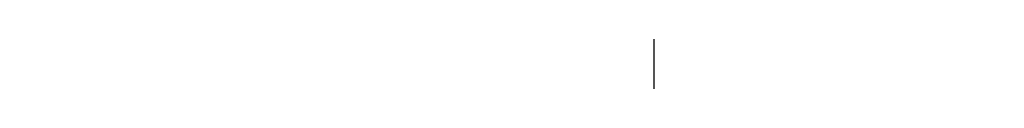
# Model space of a CAD drawing. Units: inches. Extents: x 2083 to 3317, y 1141 to 2115.
# Tile 64 of 256: x 2237.106 to 2238.294, y 1477.8 to 1477.842. Entities that reach past the tile are written whole.
import ezdxf

# ---------------------------------------------------------------- set-up
doc = ezdxf.new("R2010")
doc.units = ezdxf.units.IN
doc.layers.add('A-ANNO-DIMS', color=2, linetype='Continuous', lineweight=18)
doc.layers.add('A-WALL-PATT', color=251, linetype='Continuous', lineweight=13, true_color=0x636466)
doc.styles.get("Standard").update_dxf_attribs({"font": 'arial.ttf'})
doc.dimstyles.new('ISO-25', dxfattribs={"dimtxt": 12, "dimasz": 12, "dimexe": 1.25, "dimexo": 0.625, "dimtad": 1, "dimlunit": 3, "dimtxsty": 'Standard', "dimcen": 2.5, "dimadec": 0, "dimazin": 0, "dimtfac": 1, "dimtmove": 0, "dimatfit": 3, "dimfxl": 1, "dimarcsym": 0})

# ---------------------------------------------------------------- blocks, each defined once
blk = doc.blocks.new('*D30')
at = {"layer": 'A-ANNO-DIMS', "color": 0, "lineweight": -2, "transparency": 16777216}
for p, q in [((2240.0179, 1445.2738), (2240.0179, 1448.0455)), ((2254.3293, 1445.2738), (2254.3293, 1448.0455)), ((2228.0179, 1446.7955), (2216.0179, 1446.7955)), ((2240.0179, 1446.7955), (2254.3293, 1446.7955)), ((2266.3293, 1446.7955), (2413.7649, 1446.7955))]:
    blk.add_line(p, q, dxfattribs=at)
at = {"layer": 'A-ANNO-DIMS', "color": 0, "transparency": 16777216}
for points in [[(2228.0179, 1448.7955), (2228.0179, 1444.7955), (2240.0179, 1446.7955)], [(2266.3293, 1448.7955), (2266.3293, 1444.7955), (2254.3293, 1446.7955)]]:
    blk.add_solid(points, dxfattribs=at)
at = {"layer": 'Defpoints', "color": 0, "transparency": 16777216}
for p in [(2254.3293, 1446.7955), (2240.0179, 1444.6488), (2254.3293, 1444.6488)]:
    blk.add_point(p, dxfattribs=at)
at = {"layer": 'A-ANNO-DIMS', "color": 0, "transparency": 16777216, "insert": (2346.0471, 1453.6252), "char_height": 12, "attachment_point": 5}
blk.add_mtext('WC 1\'-2 1/2" TYP.', dxfattribs=at)
blk = doc.blocks.new('*D31')
at = {"layer": 'A-ANNO-DIMS', "color": 0, "lineweight": -2, "transparency": 16777216}
for p, q in [((2237.8711, 1456.6488), (2237.8711, 1541.9152)), ((2239.3929, 1444.6488), (2236.6211, 1444.6488)), ((2237.8711, 1431.5475), (2237.8711, 1444.6488)), ((2239.3929, 1431.5475), (2236.6211, 1431.5475)), ((2237.8711, 1419.5475), (2237.8711, 1407.5475))]:
    blk.add_line(p, q, dxfattribs=at)
at = {"layer": 'A-ANNO-DIMS', "color": 0, "transparency": 16777216}
for points in [[(2235.8711, 1456.6488), (2239.8711, 1456.6488), (2237.8711, 1444.6488)], [(2235.8711, 1419.5475), (2239.8711, 1419.5475), (2237.8711, 1431.5475)]]:
    blk.add_solid(points, dxfattribs=at)
at = {"layer": 'Defpoints', "color": 0, "transparency": 16777216}
for p in [(2237.8711, 1444.6488), (2240.0179, 1444.6488), (2240.0179, 1431.5475)]:
    blk.add_point(p, dxfattribs=at)
at = {"layer": 'A-ANNO-DIMS', "color": 0, "transparency": 16777216, "insert": (2231.2175, 1505.282), "char_height": 12, "attachment_point": 5, "rotation": 90}
blk.add_mtext('1\'-1" TYP.', dxfattribs=at)
blk = doc.blocks.new('*D45')
at = {"layer": 'A-ANNO-DIMS', "color": 0, "lineweight": -2, "transparency": 16777216}
for p, q in [((2235.9598, 1478.3864), (2235.9598, 1531.3614)), ((2418.9598, 1478.3864), (2418.9598, 1531.3614)), ((2247.9598, 1530.1114), (2406.9598, 1530.1114))]:
    blk.add_line(p, q, dxfattribs=at)
at = {"layer": 'A-ANNO-DIMS', "color": 0, "transparency": 16777216}
for points in [[(2247.9598, 1532.1114), (2247.9598, 1528.1114), (2235.9598, 1530.1114)], [(2406.9598, 1532.1114), (2406.9598, 1528.1114), (2418.9598, 1530.1114)]]:
    blk.add_solid(points, dxfattribs=at)
at = {"layer": 'Defpoints', "color": 0, "transparency": 16777216}
for p in [(2418.9598, 1530.1114), (2235.9598, 1477.7614), (2418.9598, 1477.7614)]:
    blk.add_point(p, dxfattribs=at)
at = {"layer": 'A-ANNO-DIMS', "color": 0, "transparency": 16777216, "insert": (2327.4598, 1536.8673), "char_height": 12, "attachment_point": 5}
blk.add_mtext('15\'-3"', dxfattribs=at)
blk = doc.blocks.new('*D62')
at = {"layer": 'A-ANNO-DIMS', "color": 0, "lineweight": -2, "transparency": 16777216}
for p, q in [((2235.9598, 1469.3864), (2235.9598, 1522.3614)), ((2379.9598, 1469.3864), (2379.9598, 1522.3614)), ((2247.9598, 1521.1114), (2367.9598, 1521.1114))]:
    blk.add_line(p, q, dxfattribs=at)
at = {"layer": 'A-ANNO-DIMS', "color": 0, "transparency": 16777216}
for points in [[(2247.9598, 1523.1114), (2247.9598, 1519.1114), (2235.9598, 1521.1114)], [(2367.9598, 1523.1114), (2367.9598, 1519.1114), (2379.9598, 1521.1114)]]:
    blk.add_solid(points, dxfattribs=at)
at = {"layer": 'Defpoints', "color": 0, "transparency": 16777216}
for p in [(2379.9598, 1521.1114), (2235.9598, 1468.7614), (2379.9598, 1468.7614)]:
    blk.add_point(p, dxfattribs=at)
at = {"layer": 'A-ANNO-DIMS', "color": 0, "transparency": 16777216, "insert": (2307.9598, 1527.8632), "char_height": 12, "attachment_point": 5}
blk.add_mtext('12\'-0"', dxfattribs=at)

msp = doc.modelspace()

# ---------------------------------------------------------------- hatches: boundary and pattern name
at = {"layer": 'A-WALL-PATT'}
h = msp.add_hatch(color=256, dxfattribs=at)
h.dxf.hatch_style = 1
h.paths.add_polyline_path([(3126.9598, 2020.7614), (2748.9598, 2020.7614), (2604.9598, 2020.7614), (2226.9598, 2020.7614), (2226.9598, 1702.7614), (2466.9598, 1702.7614), (2466.9598, 1582.7614), (2418.9598, 1582.7614), (2418.9598, 1477.7614), (2226.9598, 1477.7614), (2226.9598, 1263.2614), (2544.9598, 1263.2614), (2544.9598, 1411.7614), (2604.9598, 1411.7614), (2685.9598, 1411.7614), (2685.9598, 1420.7614), (2604.9598, 1420.7614), (2604.9598, 1573.7614), (2604.9598, 1702.7614), (2604.9598, 2011.7614), (2748.9598, 2011.7614), (2748.9598, 1702.7614), (2862.9598, 1702.7614), (2862.9598, 1621.7614), (2871.9598, 1621.7614), (2871.9598, 1702.7614), (2883.9598, 1702.7614), (2883.9598, 1706.9395, -0.026459), (2883.9598, 1711.7614), (2757.9598, 1711.7614), (2757.9598, 1807.7614), (2787.9598, 1807.7614), (2787.9598, 1812.2614), (2757.9598, 1812.2614), (2757.9598, 2011.7614), (2877.9598, 2011.7614), (2877.9598, 1812.2614), (2847.9598, 1812.2614), (2847.9598, 1807.7614), (2889.8357, 1807.7614), (2889.8357, 1812.2614), (2882.4598, 1812.2614), (2882.4598, 2011.7614), (3117.9598, 2011.7614), (3117.9598, 1812.2614), (2937.8357, 1812.2614), (2937.8357, 1807.7614), (2995.7098, 1807.7614), (2995.7098, 1796.1177), (3000.2098, 1796.1177), (3000.2098, 1807.7614), (3117.9598, 1807.7614), (3117.9598, 1711.7614), (3000.2098, 1711.7614), (3000.2098, 1760.1177), (2998.5727, 1760.1177, -0.020711), (2995.7098, 1760.1177), (2995.7098, 1711.7614), (2931.9598, 1711.7614), (2931.9598, 1702.7614), (3126.9598, 1702.7614)])
h.paths.add_polyline_path([(2471.4598, 2011.7614), (2471.4598, 1810.0114), (2462.7169, 1810.0114), (2462.7169, 1805.5114), (2505.9598, 1805.5114), (2505.9598, 1810.0114), (2475.9598, 1810.0114), (2475.9598, 2011.7614), (2595.9598, 2011.7614), (2595.9598, 1810.0114), (2565.9598, 1810.0114), (2565.9598, 1805.5114), (2595.9598, 1805.5114), (2595.9598, 1711.7614), (2235.9598, 1711.7614), (2235.9598, 1805.5114), (2353.7098, 1805.5114), (2353.7098, 1796.0542), (2358.2098, 1796.0542), (2358.2098, 1805.5114), (2414.7169, 1805.5114), (2414.7169, 1810.0114), (2235.9598, 1810.0114), (2235.9598, 2011.7614)], flags=16)
h.paths.add_polyline_path([(2270.2047, 1994.61), (2270.2047, 1970.61), (2246.2047, 1970.61), (2246.2047, 1994.61)], flags=0)
edge = h.paths.add_edge_path(flags=0)
edge.add_ellipse((2332.0274, 1899.7982), major_axis=(-3.043, 3.043), ratio=0.168252, start_angle=-161.3322, end_angle=-156.3071, ccw=False)
edge.add_ellipse((2333.082, 1898.7435), major_axis=(-1.0546, 1.0546), ratio=0.453532, start_angle=-123.371, end_angle=-94.1591)
edge = h.paths.add_edge_path(flags=0)
edge.add_ellipse((2332.0274, 1968.8763), major_axis=(3.043, 3.043), ratio=0.168252, start_angle=18.6678, end_angle=23.6929)
edge.add_spline(control_points=[(2332.9256, 1970.6911), (2332.2268, 1970.3361), (2330.8937, 1969.6589), (2328.4131, 1970.9321), (2327.2039, 1967.7487), (2324.7096, 1969.9556), (2322.5328, 1967.0124), (2320.0128, 1971.2958), (2317.6803, 1968.1578), (2316.0405, 1967.102), (2315.4269, 1966.8096)], knot_values=[0, 0, 0, 0, 2.267059, 4.324559, 6.685584, 8.878641, 11.121502, 14.300359, 17.755284, 19.732645, 19.732645, 19.732645, 19.732645], degree=3, periodic=0)
edge.add_ellipse((2332.0274, 1968.8763), major_axis=(3.043, 3.043), ratio=0.168252, start_angle=18.6678, end_angle=23.6929, ccw=False)
edge.add_ellipse((2333.082, 1969.9309), major_axis=(1.0546, 1.0546), ratio=0.453532, start_angle=56.629, end_angle=85.8409, ccw=False)
edge = h.paths.add_edge_path(flags=0)
edge.add_spline(control_points=[(2296.4283, 1967.9879), (2293.6278, 1965.3363), (2287.7036, 1959.7271), (2299.7439, 1949.9957), (2294.5326, 1935.6685), (2290.5732, 1920.6035), (2293.3941, 1909.9737), (2296.1854, 1904.9665)], knot_values=[0.099185, 0.099185, 0.099185, 0.099185, 0.345301, 0.619822, 0.982653, 1.386093, 1.810555, 1.810555, 1.810555, 1.810555], degree=3, periodic=0)
edge.add_spline(control_points=[(2296.1854, 1904.9665), (2297.3836, 1902.6193), (2298.001, 1901.9493), (2298.553, 1901.4682)], knot_values=[0.006246, 0.006246, 0.006246, 0.006246, 0.055476, 0.055476, 0.055476, 0.055476], degree=3, periodic=0)
edge.add_spline(control_points=[(2298.553, 1901.4682), (2297.2586, 1900.9232), (2295.2253, 1900.2321), (2293.0602, 1900.6142), (2292.1014, 1900.7884), (2292.0896, 1900.7906)], knot_values=[0.312835, 0.312835, 0.312835, 0.312835, 0.40178, 0.474987, 0.475903, 0.475903, 0.475903, 0.475903], degree=3, periodic=0)
edge.add_arc((2292.7936, 1904.6641), 3.937, 215.4209, 259.6982, ccw=False)
edge.add_spline(control_points=[(2289.5853, 1902.3823), (2289.4767, 1902.5351), (2289.3685, 1902.688), (2289.2609, 1902.8412)], knot_values=[0.102872, 0.102872, 0.102872, 0.102872, 0.116896, 0.116896, 0.116896, 0.116896], degree=3, periodic=0)
edge.add_spline(control_points=[(2289.2609, 1902.8412), (2288.6866, 1902.5502), (2287.64, 1902.0199), (2285.8813, 1901.874), (2283.853, 1901.5044), (2281.72, 1899.7105), (2278.467, 1899.4929), (2276.1571, 1901.8832), (2272.259, 1899.8041), (2267.7776, 1901.8432), (2262.2439, 1900.184), (2257.4149, 1901.7821), (2254.3184, 1900.7261), (2253.1783, 1900.3373)], knot_values=[0, 0, 0, 0, 1.907977, 3.477176, 5.261074, 7.972851, 11.680248, 13.717921, 16.939592, 22.789562, 27.502503, 33.595215, 37.145618, 37.145618, 37.145618, 37.145618], degree=3, periodic=0)
edge.add_line((2253.1783, 1900.3373), (2250.2442, 1902.8412))
edge.add_line((2250.2442, 1902.8412), (2250.2442, 1965.8333))
edge.add_line((2250.2442, 1965.8333), (2253.1783, 1968.3371))
edge.add_spline(control_points=[(2253.1783, 1968.3371), (2254.3184, 1967.9483), (2257.4149, 1966.8924), (2262.2439, 1968.4904), (2267.7776, 1966.8313), (2271.5267, 1968.5372), (2273.8759, 1967.8283), (2274.2067, 1967.7276)], knot_values=[0, 0, 0, 0, 0.09018, 0.244935, 0.364644, 0.513233, 0.537855, 0.537855, 0.537855, 0.537855], degree=3, periodic=0)
edge.add_arc((2274.3529, 1963.7933), 3.937, 72.0511, 92.1279, ccw=False)
edge.add_arc((2281.2969, 1985.23), 18.5963, 252.05113, 288.56572)
edge.add_arc((2292.3167, 1956.0289), 12.6461, 71.02679, 113.77822, ccw=False)
edge = h.paths.add_edge_path(flags=0)
edge.add_spline(control_points=[(2274.8994, 1951.8562), (2275.0662, 1951.6166), (2275.2327, 1951.3766), (2275.398, 1951.1359)], knot_values=[1.409916, 1.409916, 1.409916, 1.409916, 1.43159, 1.43159, 1.43159, 1.43159], degree=3, periodic=0)
edge.add_spline(control_points=[(2275.398, 1951.1359), (2275.7921, 1950.5619), (2276.1792, 1949.9838), (2276.5455, 1949.3971)], knot_values=[1.358238, 1.358238, 1.358238, 1.358238, 1.409916, 1.409916, 1.409916, 1.409916], degree=3, periodic=0)
edge.add_line((2276.5455, 1949.3971), (2277.4373, 1947.8622))
edge.add_spline(control_points=[(2277.4373, 1947.8622), (2276.3038, 1945.6731), (2274.6397, 1942.4269), (2274.6316, 1938.0939), (2272.7991, 1930.8515), (2274.3564, 1943.897), (2275.9477, 1947.9234), (2276.5455, 1949.3971)], knot_values=[0.005632, 0.005632, 0.005632, 0.005632, 0.186014, 0.266002, 0.357087, 0.59639, 0.739732, 0.739732, 0.739732, 0.739732], degree=3, periodic=0)
edge.add_spline(control_points=[(2276.5455, 1949.3971), (2276.1792, 1949.9838), (2275.7921, 1950.5619), (2275.398, 1951.1359)], knot_values=[1.358238, 1.358238, 1.358238, 1.358238, 1.409916, 1.409916, 1.409916, 1.409916], degree=3, periodic=0)
edge.add_spline(control_points=[(2275.398, 1951.1359), (2274.9425, 1950.0805), (2274.2078, 1948.0253), (2273.9346, 1944.8515), (2272.4685, 1937.6275), (2273.4662, 1945.6965), (2274.7006, 1951.0595), (2274.8994, 1951.8562)], knot_values=[0.104364, 0.104364, 0.104364, 0.104364, 0.189636, 0.269624, 0.36071, 0.600013, 0.644622, 0.644622, 0.644622, 0.644622], degree=3, periodic=0)
h.paths.add_polyline_path([(2269.1675, 1963.1276, -0.357527), (2268.1706, 1960.9764, -0.092561), (2268.1706, 1939.4363, -0.357527), (2269.1675, 1937.2851, -0.357527), (2267.0163, 1938.282, -0.164785), (2254.6856, 1938.282, -0.357527), (2252.5344, 1937.2851, -0.357527), (2253.5313, 1939.4363, -0.092561), (2253.5313, 1960.9764, -0.357527), (2252.5344, 1963.1276, -0.357527), (2254.6856, 1962.1307, -0.164785), (2267.0163, 1962.1307, -0.357527)], flags=0)
h.paths.add_polyline_path([(2248.8741, 1967.8018), (2248.8741, 1957.0277), (2249.4578, 1957.0277), (2249.4578, 1911.6468), (2248.8741, 1911.6468), (2248.8741, 1900.8727), (2246.5119, 1900.8727, 0.197327), (2244.1497, 1902.4569), (2244.1497, 1966.2176, 0.197327), (2246.5119, 1967.8018)], flags=0)
h.paths.add_polyline_path([(2269.1675, 1931.3893, -0.357527), (2268.1706, 1929.2381, -0.092561), (2268.1706, 1907.6981, -0.357527), (2269.1675, 1905.5469, -0.357527), (2267.0163, 1906.5438, -0.164785), (2254.6856, 1906.5438, -0.357527), (2252.5344, 1905.5469, -0.357527), (2253.5313, 1907.6981, -0.092561), (2253.5313, 1929.2381, -0.357527), (2252.5344, 1931.3893, -0.357527), (2254.6856, 1930.3925, -0.164785), (2267.0163, 1930.3925, -0.357527)], flags=0)
edge = h.paths.add_edge_path(flags=0)
edge.add_spline(control_points=[(2276.1969, 1906.7237), (2276.1681, 1909.0289), (2276.114, 1913.3719), (2270.5984, 1924.925), (2273.9052, 1919.0128), (2275.9217, 1916.2621), (2275.4746, 1912.4021), (2277.2579, 1910.3806), (2276.696, 1908.225), (2276.6462, 1906.813), (2276.6178, 1906.0084)], knot_values=[0, 0, 0, 0, 8.61026, 16.221274, 18.843057, 23.804898, 27.440828, 29.356102, 31.203478, 33.650687, 33.650687, 33.650687, 33.650687], degree=3, periodic=0)
edge.add_spline(control_points=[(2276.6178, 1906.0084), (2276.6233, 1905.6241), (2276.4977, 1904.6287), (2275.4418, 1903.8547), (2274.9373, 1903.0804), (2274.8591, 1902.8412)], knot_values=[0.156488, 0.156488, 0.156488, 0.156488, 0.184398, 0.231376, 0.250598, 0.250598, 0.250598, 0.250598], degree=3, periodic=0)
edge.add_line((2274.8591, 1902.8412), (2276.506, 1902.8412))
edge.add_spline(control_points=[(2276.506, 1902.8412), (2276.7883, 1903.0849), (2277.6651, 1904.1252), (2278.2495, 1904.3407), (2277.6539, 1908.5274), (2278.1557, 1906.2278), (2278.1005, 1905.2859), (2278.8467, 1904.069), (2277.8568, 1903.4149), (2277.8742, 1902.991), (2277.9036, 1902.8412)], knot_values=[0.059574, 0.059574, 0.059574, 0.059574, 0.080753, 0.103741, 0.16972, 0.176036, 0.207137, 0.240474, 0.262341, 0.27366, 0.27366, 0.27366, 0.27366], degree=3, periodic=0)
edge.add_line((2277.9036, 1902.8412), (2280.0298, 1902.8412))
edge.add_spline(control_points=[(2280.0298, 1902.8412), (2279.8882, 1903.0884), (2279.4993, 1903.9816), (2280.1523, 1905.9393), (2278.1036, 1909.6578), (2279.7624, 1907.1853), (2280.3279, 1904.8749), (2280.4851, 1903.4896), (2281.4633, 1903.2494), (2281.7583, 1902.9365), (2281.834, 1902.8412)], knot_values=[0.013856, 0.013856, 0.013856, 0.013856, 0.034874, 0.088867, 0.107879, 0.126738, 0.158714, 0.193757, 0.217487, 0.226722, 0.226722, 0.226722, 0.226722], degree=3, periodic=0)
edge.add_spline(control_points=[(2281.834, 1902.8412), (2281.7875, 1902.8267), (2281.647, 1902.783), (2281.3955, 1902.8595), (2281.0881, 1902.9852), (2280.7207, 1903.0609), (2280.3335, 1903.0257), (2280.1248, 1902.8989), (2280.0298, 1902.8412)], knot_values=[0, 0, 0, 0, 0.14413, 0.435517, 0.749276, 1.153046, 1.548371, 1.878348, 1.878348, 1.878348, 1.878348], degree=3, periodic=0)
edge.add_line((2280.0298, 1902.8412), (2277.9036, 1902.8412))
edge.add_spline(control_points=[(2277.9036, 1902.8412), (2277.8929, 1902.7959), (2277.8654, 1902.6796), (2277.6075, 1902.6875), (2277.2741, 1902.8007), (2276.8379, 1902.6198), (2276.5838, 1902.7893), (2276.506, 1902.8412)], knot_values=[0, 0, 0, 0, 0.127189, 0.326199, 0.628009, 1.24357, 1.515331, 1.515331, 1.515331, 1.515331], degree=3, periodic=0)
edge.add_line((2276.506, 1902.8412), (2274.8591, 1902.8412))
edge.add_spline(control_points=[(2274.8591, 1902.8412), (2274.8144, 1902.8986), (2274.7251, 1903.0134), (2274.4935, 1903.119), (2274.2443, 1902.9605), (2273.9371, 1903.1849), (2273.614, 1902.9831), (2273.4083, 1902.883), (2273.3223, 1902.8412)], knot_values=[0, 0, 0, 0, 0.21843, 0.436957, 0.687977, 0.990379, 1.398396, 1.69185, 1.69185, 1.69185, 1.69185], degree=3, periodic=0)
edge.add_spline(control_points=[(2273.3223, 1902.8412), (2273.6167, 1903.4457), (2274.274, 1904.5383), (2276.0272, 1904.5737), (2276.207, 1906.5836), (2276.1969, 1906.7237)], knot_values=[0.012227, 0.012227, 0.012227, 0.012227, 0.059472, 0.106218, 0.134458, 0.134458, 0.134458, 0.134458], degree=3, periodic=0)
h.paths.add_polyline_path([(2270.7761, 1897.7898), (2270.7761, 1873.7898), (2246.7761, 1873.7898), (2246.7761, 1897.7898)], flags=0)
h.paths.add_polyline_path([(2353.7098, 1760.0051), (2353.7098, 1760.0542), (2358.2098, 1760.0542, -0.033729)], flags=0)
h.paths.add_polyline_path([(2321.8191, 1737.5292), (2341.9953, 1737.5292, -0.414214), (2343.2033, 1736.3212), (2343.2033, 1721.0206, -0.414214), (2341.9953, 1719.8127), (2321.8191, 1719.8127, -0.414214), (2320.6112, 1721.0206), (2320.6112, 1736.3212, -0.414214)], flags=0)
h.paths.add_polyline_path([(2324.235, 1736.3212), (2339.5794, 1736.3212, -0.414214), (2341.9953, 1733.9053), (2341.9953, 1725.4497, -0.414214), (2339.5794, 1723.0338), (2333.6806, 1723.0338), (2333.8453, 1722.0455, -0.870646), (2335.4254, 1721.8259, -0.767327), (2333.9227, 1721.4232), (2331.291, 1721.4232, -0.767327), (2329.7883, 1721.8259, -0.870646), (2331.3684, 1722.0455), (2331.5331, 1723.0338), (2324.235, 1723.0338, -0.414214), (2321.8191, 1725.4497), (2321.8191, 1733.9053, -0.414214)], flags=0)
h.paths.add_polyline_path([(2570.4838, 1928.6154), (2589.6838, 1928.6154), (2590.1688, 1928.6154), (2590.1688, 1904.9934), (2570.4838, 1904.9934)], flags=0)
h.paths.add_polyline_path([(2574.4473, 1927.2638, -1), (2572.8288, 1927.2638, -1)], flags=0)
h.paths.add_polyline_path([(2573.0899, 1926.9409), (2573.925, 1927.776), (2574.1477, 1927.5533), (2573.3126, 1926.7182)], flags=0)
h.paths.add_polyline_path([(2578.7791, 1919.7296, -1), (2571.5917, 1919.7296, -1)], flags=0)
h.paths.add_polyline_path([(2578.3854, 1919.7296, -1), (2571.9854, 1919.7296, -1)], flags=0)
h.paths.add_polyline_path([(2331.5958, 1729.4762, -1), (2333.618, 1729.4762, -1)], flags=0)
h.paths.add_polyline_path([(2578.0342, 1927.2638, -1), (2576.4157, 1927.2638, -1)], flags=0)
h.paths.add_polyline_path([(2576.6889, 1927.5311), (2576.9116, 1927.7538), (2577.7467, 1926.9186), (2577.524, 1926.6959)], flags=0)
h.paths.add_polyline_path([(2578.1391, 1909.8595, -1), (2572.2317, 1909.8595, -1)], flags=0)
h.paths.add_polyline_path([(2577.7454, 1909.8595, -1), (2572.6254, 1909.8595, -1)], flags=0)
h.paths.add_polyline_path([(2583.7977, 1927.2638, -1), (2582.1792, 1927.2638, -1)], flags=0)
h.paths.add_polyline_path([(2582.7186, 1927.7538), (2583.5538, 1926.9186), (2583.3311, 1926.6959), (2582.4959, 1927.5311)], flags=0)
h.paths.add_polyline_path([(2582.4959, 1927.5311), (2582.7186, 1927.7538), (2583.5538, 1926.9186), (2583.3311, 1926.6959)], flags=0)
h.paths.add_polyline_path([(2587.7391, 1920.5296, -1), (2581.8317, 1920.5296, -1)], flags=0)
h.paths.add_polyline_path([(2587.3454, 1920.5296, -1), (2582.2254, 1920.5296, -1)], flags=0)
h.paths.add_polyline_path([(2587.3846, 1927.2638, -1), (2585.7661, 1927.2638, -1)], flags=0)
h.paths.add_polyline_path([(2586.082, 1926.9802), (2586.9172, 1927.8154), (2587.1399, 1927.5927), (2586.3047, 1926.7575)], flags=0)
h.paths.add_polyline_path([(2588.3791, 1910.6595, -1), (2581.1917, 1910.6595, -1)], flags=0)
h.paths.add_polyline_path([(2587.9854, 1910.6595, -1), (2581.5854, 1910.6595, -1)], flags=0)
h.paths.add_polyline_path([(2417.1677, 1729.4779), (2437.3439, 1729.4779, -0.414214), (2438.5519, 1728.2699), (2438.5519, 1712.9693, -0.414214), (2437.3439, 1711.7614), (2417.1677, 1711.7614, -0.414214), (2415.9598, 1712.9693), (2415.9598, 1728.2699, -0.414214)], flags=0)
h.paths.add_polyline_path([(2419.5836, 1728.2699), (2434.928, 1728.2699, -0.414214), (2437.3439, 1725.8541), (2437.3439, 1717.3984, -0.414214), (2434.928, 1714.9825), (2429.0292, 1714.9825), (2429.1939, 1713.9942, -0.870646), (2430.774, 1713.7746, -0.767327), (2429.2713, 1713.372), (2426.6396, 1713.372, -0.767327), (2425.1369, 1713.7746, -0.870646), (2426.717, 1713.9942), (2426.8817, 1714.9825), (2419.5836, 1714.9825, -0.414214), (2417.1677, 1717.3984), (2417.1677, 1725.8541, -0.414214)], flags=0)
h.paths.add_polyline_path([(2419.5836, 1728.2699), (2434.928, 1728.2699, -0.414214), (2437.3439, 1725.8541), (2437.3439, 1717.3984, -0.414214), (2434.928, 1714.9825), (2429.0292, 1714.9825), (2428.3581, 1719.009), (2427.5528, 1719.009), (2426.8817, 1714.9825), (2419.5836, 1714.9825, -0.414214), (2417.1677, 1717.3984), (2417.1677, 1725.8541, -0.414214)], flags=0)
h.paths.add_polyline_path([(2426.9444, 1721.4249, -1), (2428.9666, 1721.4249, -1)], flags=0)
h.paths.add_polyline_path([(2475.9598, 1702.7614), (2595.9598, 1702.7614), (2595.9598, 1582.7614), (2475.9598, 1582.7614)], flags=16)
h.paths.add_polyline_path([(2427.9598, 1573.7614), (2595.9598, 1573.7614), (2595.9598, 1468.7614), (2595.9598, 1420.7614), (2384.4598, 1420.7614), (2384.4598, 1468.7614), (2427.9598, 1468.7614)], flags=16)
h.paths.add_polyline_path([(2379.9598, 1468.7614), (2379.9598, 1420.7614), (2235.9598, 1420.7614), (2235.9598, 1468.7614)], flags=16)
h.paths.add_polyline_path([(2317.816, 1466.6958), (2337.9922, 1466.6958, -0.414214), (2339.2002, 1465.4878), (2339.2002, 1450.1872, -0.414214), (2337.9922, 1448.9792), (2317.816, 1448.9792, -0.414214), (2316.6081, 1450.1872), (2316.6081, 1465.4878, -0.414214)], flags=0)
h.paths.add_polyline_path([(2320.2319, 1465.4878), (2335.5763, 1465.4878, -0.414214), (2337.9922, 1463.0719), (2337.9922, 1454.6163, -0.414214), (2335.5763, 1452.2004), (2329.6775, 1452.2004), (2329.8422, 1451.212, -0.870646), (2331.4223, 1450.9925, -0.767327), (2329.9196, 1450.5898), (2327.2879, 1450.5898, -0.767327), (2325.7852, 1450.9925, -0.870646), (2327.3653, 1451.212), (2327.53, 1452.2004), (2320.2319, 1452.2004, -0.414214), (2317.816, 1454.6163), (2317.816, 1463.0719, -0.414214)], flags=0)
h.paths.add_polyline_path([(2320.2319, 1465.4878), (2335.5763, 1465.4878, -0.414214), (2337.9922, 1463.0719), (2337.9922, 1454.6163, -0.414214), (2335.5763, 1452.2004), (2329.6775, 1452.2004), (2329.0064, 1456.2269), (2328.2011, 1456.2269), (2327.53, 1452.2004), (2320.2319, 1452.2004, -0.414214), (2317.816, 1454.6163), (2317.816, 1463.0719, -0.414214)], flags=0)
h.paths.add_polyline_path([(2327.5926, 1458.6428, -1), (2329.6148, 1458.6428, -1)], flags=0)
h.paths.add_polyline_path([(2244.4117, 1433.3405), (2241.9209, 1433.3405, -0.414214), (2240.0179, 1435.2435), (2240.0179, 1440.9528, -0.414211), (2241.9209, 1442.8559), (2244.4117, 1442.8559, -1.976472)], flags=0)
h.paths.add_polyline_path([(2245.3569, 1434.3975, -0.414214), (2245.3569, 1441.7988, -2.144098)], flags=0)
h.paths.add_polyline_path([(2535.9598, 1416.2614), (2535.9598, 1272.2614), (2235.9598, 1272.2614), (2235.9598, 1416.2614)], flags=16)
h.paths.add_polyline_path([(2260.1196, 1384.2928), (2260.1196, 1362.0386), (2237.8654, 1362.0386), (2237.8654, 1384.2928)], flags=0)
edge = h.paths.add_edge_path(flags=0)
edge.add_line((2318.2518, 1362.0933), (2318.1458, 1362.001))
edge.add_ellipse((2317.4451, 1360.431), major_axis=(2.8216, 2.8216), ratio=0.168252, start_angle=18.6678, end_angle=20.9481, ccw=False)
edge.add_ellipse((2318.423, 1361.409), major_axis=(0.9779, 0.9779), ratio=0.453532, start_angle=56.629, end_angle=70.2262, ccw=False)
edge = h.paths.add_edge_path(flags=0)
edge.add_line((2319.1074, 1295.5711), (2319.015, 1295.6771))
edge.add_ellipse((2317.4451, 1296.3778), major_axis=(-2.8216, 2.8216), ratio=0.168252, start_angle=-161.3322, end_angle=-159.0519, ccw=False)
edge.add_ellipse((2318.423, 1295.3999), major_axis=(-0.9779, 0.9779), ratio=0.453532, start_angle=-123.371, end_angle=-109.7738)
edge = h.paths.add_edge_path(flags=0)
edge.add_spline(control_points=[(2284.2103, 1301.1702), (2284.5807, 1300.4447), (2284.8912, 1299.892), (2285.1596, 1299.461)], knot_values=[0.039066, 0.039066, 0.039066, 0.039066, 0.055476, 0.055476, 0.055476, 0.055476], degree=3, periodic=0)
edge.add_line((2285.1596, 1299.461), (2284.2103, 1301.1702))
edge = h.paths.add_edge_path(flags=0)
edge.add_line((2280.4125, 1297.298), (2283.37, 1297.0361))
edge.add_line((2283.37, 1297.0361), (2286.4057, 1297.9263))
edge.add_spline(control_points=[(2286.4057, 1297.9263), (2285.3055, 1297.4631), (2284.3448, 1297.1292), (2283.37, 1297.0361)], knot_values=[0.394369, 0.394369, 0.394369, 0.394369, 0.475903, 0.475903, 0.475903, 0.475903], degree=3, periodic=0)
edge.add_spline(control_points=[(2283.37, 1297.0361), (2283.2814, 1297.0277), (2282.3163, 1296.9573), (2281.3125, 1297.1345), (2280.4234, 1297.296), (2280.4125, 1297.298)], knot_values=[0.312835, 0.312835, 0.312835, 0.312835, 0.320246, 0.393453, 0.394369, 0.394369, 0.394369, 0.394369], degree=3, periodic=0)
edge = h.paths.add_edge_path(flags=0)
edge.add_line((2284.4356, 1359.6073), (2280.4463, 1355.328))
edge.add_line((2280.4463, 1355.328), (2279.58, 1351.0178))
edge.add_line((2279.58, 1351.0178), (2282.413, 1346.5804))
edge.add_spline(control_points=[(2282.413, 1346.5804), (2283.1533, 1345.5892), (2284.2529, 1344.0289), (2284.801, 1342.3872), (2284.9352, 1341.8055)], knot_values=[1.240098, 1.240098, 1.240098, 1.240098, 1.332892, 1.382712, 1.382712, 1.382712, 1.382712], degree=3, periodic=0)
edge.add_spline(control_points=[(2284.9352, 1341.8055), (2285.3191, 1340.1406), (2285.233, 1338.4092), (2284.9099, 1336.6541)], knot_values=[1.097484, 1.097484, 1.097484, 1.097484, 1.240098, 1.240098, 1.240098, 1.240098], degree=3, periodic=0)
edge.add_spline(control_points=[(2284.9099, 1336.6541), (2284.5868, 1334.899), (2284.0267, 1333.1203), (2283.4626, 1331.3606)], knot_values=[0.95487, 0.95487, 0.95487, 0.95487, 1.097484, 1.097484, 1.097484, 1.097484], degree=3, periodic=0)
edge.add_line((2283.4626, 1331.3606), (2281.8904, 1326.1534))
edge.add_line((2281.8904, 1326.1534), (2280.7563, 1321.0561))
edge.add_line((2280.7563, 1321.0561), (2280.2992, 1316.002))
edge.add_line((2280.2992, 1316.002), (2280.7159, 1310.9501))
edge.add_line((2280.7159, 1310.9501), (2282.0281, 1305.9721))
edge.add_line((2282.0281, 1305.9721), (2284.2103, 1301.1702))
edge.add_spline(control_points=[(2284.2103, 1301.1702), (2283.3407, 1302.7302), (2282.6119, 1304.3365), (2282.0281, 1305.9721)], knot_values=[0.099185, 0.099185, 0.099185, 0.099185, 0.241799, 0.241799, 0.241799, 0.241799], degree=3, periodic=0)
edge.add_spline(control_points=[(2282.0281, 1305.9721), (2281.4443, 1307.6078), (2281.0055, 1309.2728), (2280.7159, 1310.9501)], knot_values=[0.241799, 0.241799, 0.241799, 0.241799, 0.384413, 0.384413, 0.384413, 0.384413], degree=3, periodic=0)
edge.add_spline(control_points=[(2280.7159, 1310.9501), (2280.4332, 1312.5876), (2280.2894, 1314.277), (2280.2989, 1315.962), (2280.2992, 1316.002)], knot_values=[0.384413, 0.384413, 0.384413, 0.384413, 0.523647, 0.527028, 0.527028, 0.527028, 0.527028], degree=3, periodic=0)
edge.add_spline(control_points=[(2280.2992, 1316.002), (2280.3123, 1317.687), (2280.4779, 1319.3679), (2280.7563, 1321.0561)], knot_values=[0.527028, 0.527028, 0.527028, 0.527028, 0.669642, 0.669642, 0.669642, 0.669642], degree=3, periodic=0)
edge.add_spline(control_points=[(2280.7563, 1321.0561), (2281.0346, 1322.7443), (2281.4259, 1324.4396), (2281.8904, 1326.1534)], knot_values=[0.669642, 0.669642, 0.669642, 0.669642, 0.812256, 0.812256, 0.812256, 0.812256], degree=3, periodic=0)
edge.add_spline(control_points=[(2281.8904, 1326.1534), (2282.2644, 1327.5333), (2282.7879, 1329.2618), (2283.3528, 1331.0178), (2283.4626, 1331.3606)], knot_values=[0.812256, 0.812256, 0.812256, 0.812256, 0.927087, 0.95487, 0.95487, 0.95487, 0.95487], degree=3, periodic=0)
edge.add_line((2283.4626, 1331.3606), (2284.9099, 1336.6541))
edge.add_line((2284.9099, 1336.6541), (2284.9352, 1341.8055))
edge.add_line((2284.9352, 1341.8055), (2282.413, 1346.5804))
edge.add_spline(control_points=[(2282.413, 1346.5804), (2281.2751, 1348.1038), (2280.0784, 1349.5703), (2279.58, 1351.0178)], knot_values=[1.382712, 1.382712, 1.382712, 1.382712, 1.525326, 1.525326, 1.525326, 1.525326], degree=3, periodic=0)
edge.add_spline(control_points=[(2279.58, 1351.0178), (2279.4433, 1351.4147), (2279.1363, 1352.8569), (2279.7352, 1354.2904), (2280.4463, 1355.328)], knot_values=[1.525326, 1.525326, 1.525326, 1.525326, 1.564439, 1.667941, 1.667941, 1.667941, 1.667941], degree=3, periodic=0)
edge.add_spline(control_points=[(2280.4463, 1355.328), (2281.4261, 1356.7578), (2282.9308, 1358.1826), (2284.4356, 1359.6073)], knot_values=[1.667941, 1.667941, 1.667941, 1.667941, 1.810555, 1.810555, 1.810555, 1.810555], degree=3, periodic=0)
edge.add_arc((2280.6231, 1348.5182), 11.7262, 71.02679, 113.77822)
edge.add_arc((2270.4049, 1375.5952), 17.2436, 252.05113, 288.56572, ccw=False)
edge.add_arc((2263.966, 1355.7178), 3.6506, 72.0511, 92.1279)
edge.add_arc((2263.966, 1355.7178), 3.6506, 92.1279, 177.9851)
edge.add_spline(control_points=[(2260.3176, 1355.8462), (2260.2604, 1354.2207), (2260.5513, 1350.1865), (2262.9993, 1346.7663), (2264.4727, 1344.649)], knot_values=[1.43159, 1.43159, 1.43159, 1.43159, 1.564144, 1.770695, 1.770695, 1.770695, 1.770695], degree=3, periodic=0)
edge.add_line((2264.4727, 1344.649), (2264.9356, 1343.9825))
edge.add_spline(control_points=[(2263.801, 1340.2481), (2263.8432, 1340.5141), (2264.0672, 1341.7565), (2264.5127, 1343.0025), (2264.935, 1343.9811)], knot_values=[0.53657, 0.53657, 0.53657, 0.53657, 0.559349, 0.644622, 0.644622, 0.644622, 0.644622], degree=3, periodic=0)
edge.add_spline(control_points=[(2264.935, 1343.9811), (2265.1178, 1343.715), (2265.2989, 1343.4479), (2265.4768, 1343.1794)], knot_values=[1.384077, 1.384077, 1.384077, 1.384077, 1.409916, 1.409916, 1.409916, 1.409916], degree=3, periodic=0)
edge.add_spline(control_points=[(2265.4768, 1343.1794), (2265.6546, 1342.9108), (2265.8293, 1342.6408), (2265.9991, 1342.3688)], knot_values=[1.358238, 1.358238, 1.358238, 1.358238, 1.384077, 1.384077, 1.384077, 1.384077], degree=3, periodic=0)
edge.add_line((2265.9991, 1342.3688), (2266.826, 1340.9455))
edge.add_spline(control_points=[(2266.826, 1340.9455), (2268.8944, 1337.0897), (2271.3982, 1325.843), (2270.5162, 1310.5686), (2275.9194, 1301.8606), (2277.7895, 1299.1994)], knot_values=[0.116896, 0.116896, 0.116896, 0.116896, 0.472987, 1.050969, 1.313793, 1.313793, 1.313793, 1.313793], degree=3, periodic=0)
edge.add_spline(control_points=[(2277.7895, 1299.1994), (2277.8394, 1299.1285), (2277.8894, 1299.0575), (2277.9396, 1298.9866)], knot_values=[0.109884, 0.109884, 0.109884, 0.109884, 0.116896, 0.116896, 0.116896, 0.116896], degree=3, periodic=0)
edge.add_line((2277.9396, 1298.9866), (2277.7888, 1299.1991))
edge.add_spline(control_points=[(2277.7888, 1299.1991), (2277.2566, 1298.9294), (2276.2864, 1298.4379), (2275.0394, 1298.3344), (2274.3833, 1298.2389), (2274.2153, 1298.2093)], knot_values=[33.12187, 33.12187, 33.12187, 33.12187, 35.029056, 36.598255, 37.144827, 37.144827, 37.144827, 37.144827], degree=3, periodic=0)
edge.add_line((2274.2153, 1298.2093), (2273.0731, 1297.893))
edge.add_spline(control_points=[(2273.0731, 1297.893), (2272.3229, 1297.5798), (2271.0392, 1296.5105), (2269.2484, 1296.2261), (2268.4231, 1296.3747)], knot_values=[26.532584, 26.532584, 26.532584, 26.532584, 29.198919, 31.839101, 31.839101, 31.839101, 31.839101], degree=3, periodic=0)
edge.add_line((2268.4231, 1296.3747), (2263.8785, 1297.4575))
edge.add_spline(control_points=[(2263.8785, 1297.4575), (2263.5561, 1297.3594), (2261.8603, 1296.8387), (2260.2388, 1297.2824), (2258.9335, 1297.5165)], knot_values=[15.919551, 15.919551, 15.919551, 15.919551, 16.939592, 21.226067, 21.226067, 21.226067, 21.226067], degree=3, periodic=0)
edge.add_line((2258.9335, 1297.5165), (2254.0552, 1297.329))
edge.add_spline(control_points=[(2254.0552, 1297.329), (2253.7555, 1297.2958), (2252.1137, 1297.1652), (2250.4619, 1297.5442), (2249.1297, 1297.6679)], knot_values=[5.306517, 5.306517, 5.306517, 5.306517, 6.276435, 10.613034, 10.613034, 10.613034, 10.613034], degree=3, periodic=0)
edge.add_line((2249.1297, 1297.6679), (2244.3316, 1296.8778))
edge.add_line((2244.3316, 1296.8778), (2241.611, 1299.1994))
edge.add_line((2241.611, 1299.1994), (2241.611, 1357.6094))
edge.add_line((2241.611, 1357.6094), (2244.3316, 1359.9311))
edge.add_line((2244.3316, 1359.9311), (2252.7288, 1359.5427))
edge.add_spline(control_points=[(2252.7288, 1359.5427), (2252.8709, 1359.5464), (2253.3057, 1359.5482), (2253.7398, 1359.5143), (2254.0317, 1359.4824)], knot_values=[0.233291, 0.233291, 0.233291, 0.233291, 0.244935, 0.268927, 0.268927, 0.268927, 0.268927], degree=3, periodic=0)
edge.add_line((2254.0317, 1359.4824), (2259.5872, 1359.4164))
edge.add_spline(control_points=[(2259.5872, 1359.4164), (2260.6771, 1359.6285), (2262.0732, 1359.897), (2263.5237, 1359.4593), (2263.8304, 1359.366)], knot_values=[0.422516, 0.422516, 0.422516, 0.422516, 0.513233, 0.537855, 0.537855, 0.537855, 0.537855], degree=3, periodic=0)
edge.add_arc((2263.966, 1355.7178), 3.6506, 72.0511, 92.1279, ccw=False)
edge.add_arc((2270.4049, 1375.5952), 17.2436, 252.05113, 288.56572)
edge.add_arc((2280.6231, 1348.5182), 11.7262, 71.02679, 113.77822, ccw=False)
h.paths.add_polyline_path([(2240.3405, 1359.4347), (2240.3405, 1349.4444), (2240.8818, 1349.4444), (2240.8818, 1307.3645), (2240.3405, 1307.3645), (2240.3405, 1297.3741), (2238.1502, 1297.3741, 0.197327), (2235.9598, 1298.8431), (2235.9598, 1357.9657, 0.197327), (2238.1502, 1359.4347)], flags=0)
h.paths.add_polyline_path([(2259.1578, 1355.1005, -0.357527), (2258.2334, 1353.1058, -0.092561), (2258.2334, 1333.1326, -0.357527), (2259.1578, 1331.1379, -0.357527), (2257.1631, 1332.0622, -0.164785), (2245.7293, 1332.0622, -0.357527), (2243.7346, 1331.1379, -0.357527), (2244.6589, 1333.1326, -0.092561), (2244.6589, 1353.1058, -0.357527), (2243.7346, 1355.1005, -0.357527), (2245.7293, 1354.1761, -0.164785), (2257.1631, 1354.1761, -0.357527)], flags=0)
edge = h.paths.add_edge_path(flags=0)
edge.add_line((2265.9991, 1342.3688), (2266.826, 1340.9455))
edge.add_line((2266.826, 1340.9455), (2265.3076, 1337.8141))
edge.add_line((2265.3076, 1337.8141), (2264.3582, 1334.6529))
edge.add_line((2264.3582, 1334.6529), (2264.262, 1333.7997))
edge.add_spline(control_points=[(2264.262, 1333.7997), (2264.2084, 1333.1871), (2264.1621, 1332.3655), (2264.0071, 1331.4139), (2263.969, 1331.2018)], knot_values=[0.464444, 0.464444, 0.464444, 0.464444, 0.516691, 0.531608, 0.531608, 0.531608, 0.531608], degree=3, periodic=0)
edge.add_spline(control_points=[(2263.969, 1331.2018), (2263.7745, 1330.1189), (2263.4244, 1328.7908), (2263.2574, 1328.5307), (2263.234, 1328.5146)], knot_values=[0.372682, 0.372682, 0.372682, 0.372682, 0.44885, 0.464444, 0.464444, 0.464444, 0.464444], degree=3, periodic=0)
edge.add_spline(control_points=[(2263.234, 1328.5146), (2263.0964, 1328.4202), (2263.1312, 1329.3015), (2263.275, 1330.6157)], knot_values=[0.280919, 0.280919, 0.280919, 0.280919, 0.372682, 0.372682, 0.372682, 0.372682], degree=3, periodic=0)
edge.add_spline(control_points=[(2263.275, 1330.6157), (2263.4187, 1331.93), (2263.6715, 1333.6773), (2263.9699, 1335.315)], knot_values=[0.189157, 0.189157, 0.189157, 0.189157, 0.280919, 0.280919, 0.280919, 0.280919], degree=3, periodic=0)
edge.add_spline(control_points=[(2263.9699, 1335.315), (2264.1005, 1336.0322), (2264.4188, 1337.6219), (2264.7548, 1338.8644), (2264.9474, 1339.4911)], knot_values=[0.097394, 0.097394, 0.097394, 0.097394, 0.137578, 0.189157, 0.189157, 0.189157, 0.189157], degree=3, periodic=0)
edge.add_spline(control_points=[(2264.9474, 1339.4911), (2265.29, 1340.6061), (2265.6442, 1341.494), (2265.9991, 1342.3688)], knot_values=[0.005632, 0.005632, 0.005632, 0.005632, 0.097394, 0.097394, 0.097394, 0.097394], degree=3, periodic=0)
h.paths.add_polyline_path([(2259.1578, 1325.671, -0.357527), (2258.2334, 1323.6763, -0.092561), (2258.2334, 1303.7031, -0.357527), (2259.1578, 1301.7084, -0.357527), (2257.1631, 1302.6327, -0.164785), (2245.7293, 1302.6327, -0.357527), (2243.7346, 1301.7084, -0.357527), (2244.6589, 1303.7031, -0.092561), (2244.6589, 1323.6763, -0.357527), (2243.7346, 1325.671, -0.357527), (2245.7293, 1324.7466, -0.164785), (2257.1631, 1324.7466, -0.357527)], flags=0)
edge = h.paths.add_edge_path(flags=0)
edge.add_spline(control_points=[(2261.7089, 1317.3114), (2261.6795, 1317.4176), (2261.7619, 1317.3885), (2262.4907, 1316.0899), (2262.9622, 1315.3009)], knot_values=[14.955861, 14.955861, 14.955861, 14.955861, 16.221274, 18.694826, 18.694826, 18.694826, 18.694826], degree=3, periodic=0)
edge.add_spline(control_points=[(2262.9622, 1315.3009), (2262.9904, 1315.2536), (2263.7021, 1314.0674), (2264.349, 1313.1272), (2264.7301, 1312.1642)], knot_values=[18.694826, 18.694826, 18.694826, 18.694826, 18.843057, 22.433791, 22.433791, 22.433791, 22.433791], degree=3, periodic=0)
edge.add_spline(control_points=[(2264.7301, 1312.1642), (2264.8756, 1311.7964), (2265.1769, 1310.7698), (2265.1431, 1309.5593), (2265.2477, 1308.8242)], knot_values=[22.433791, 22.433791, 22.433791, 22.433791, 23.804898, 26.172756, 26.172756, 26.172756, 26.172756], degree=3, periodic=0)
edge.add_line((2265.2477, 1308.8242), (2265.8508, 1307.1719))
edge.add_spline(control_points=[(2265.8508, 1307.1719), (2266.065, 1306.8217), (2266.3844, 1306.3322), (2266.4244, 1305.7805), (2266.4204, 1305.6112)], knot_values=[28.062562, 28.062562, 28.062562, 28.062562, 29.356102, 29.911721, 29.911721, 29.911721, 29.911721], degree=3, periodic=0)
edge.add_spline(control_points=[(2266.4204, 1305.6112), (2266.4161, 1305.4326), (2266.394, 1305.25), (2266.3648, 1305.0659)], knot_values=[29.911721, 29.911721, 29.911721, 29.911721, 30.497837, 30.497837, 30.497837, 30.497837], degree=3, periodic=0)
edge.add_line((2266.3648, 1305.0659), (2266.0662, 1302.1363))
edge.add_spline(control_points=[(2266.0662, 1302.1363), (2266.0712, 1301.78), (2265.9981, 1301.2), (2265.6633, 1300.759), (2265.5089, 1300.5859)], knot_values=[0.156488, 0.156488, 0.156488, 0.156488, 0.184398, 0.203543, 0.203543, 0.203543, 0.203543], degree=3, periodic=0)
edge.add_line((2265.5089, 1300.5859), (2264.4353, 1299.1994))
edge.add_line((2264.4353, 1299.1994), (2265.9624, 1299.1994))
edge.add_line((2265.9624, 1299.1994), (2267.336, 1301.1753))
edge.add_line((2267.336, 1301.1753), (2267.3117, 1301.9862))
edge.add_spline(control_points=[(2267.3117, 1301.9862), (2267.2611, 1302.8624), (2267.1602, 1303.7371), (2267.2715, 1303.3259)], knot_values=[0.126229, 0.126229, 0.126229, 0.126229, 0.166617, 0.166617, 0.166617, 0.166617], degree=3, periodic=0)
edge.add_spline(control_points=[(2267.2715, 1303.3259), (2267.28, 1303.2943), (2267.3098, 1303.1754), (2267.3735, 1302.8836), (2267.4061, 1302.6828), (2267.4179, 1302.601)], knot_values=[0.166617, 0.166617, 0.166617, 0.166617, 0.16972, 0.176036, 0.180765, 0.180765, 0.180765, 0.180765], degree=3, periodic=0)
edge.add_spline(control_points=[(2267.7439, 1300.9875), (2267.6876, 1301.1509), (2267.4805, 1301.6567), (2267.4838, 1302.1448), (2267.4179, 1302.601)], knot_values=[0.180765, 0.180765, 0.180765, 0.180765, 0.193767, 0.220139, 0.220139, 0.220139, 0.220139], degree=3, periodic=0)
edge.add_line((2267.4179, 1302.601), (2267.7439, 1300.9875))
edge.add_spline(control_points=[(2267.7439, 1300.9875), (2267.832, 1300.7319), (2267.932, 1300.3099), (2267.5548, 1299.9745), (2267.4294, 1299.8292)], knot_values=[0.220139, 0.220139, 0.220139, 0.220139, 0.240474, 0.25489, 0.25489, 0.25489, 0.25489], degree=3, periodic=0)
edge.add_line((2267.4294, 1299.8292), (2267.2584, 1299.1994))
edge.add_line((2267.2584, 1299.1994), (2269.23, 1299.1994))
edge.add_spline(control_points=[(2269.23, 1299.1994), (2269.0987, 1299.4287), (2268.8428, 1300.0163), (2269.0116, 1300.9159), (2268.9468, 1301.6607)], knot_values=[0.013856, 0.013856, 0.013856, 0.013856, 0.034874, 0.067073, 0.067073, 0.067073, 0.067073], degree=3, periodic=0)
edge.add_line((2268.9468, 1301.6607), (2268.4316, 1303.6031))
edge.add_spline(control_points=[(2268.4316, 1303.6031), (2268.1756, 1304.1924), (2267.5962, 1305.2513), (2268.0407, 1304.6232), (2268.2514, 1304.2824)], knot_values=[0.090155, 0.090155, 0.090155, 0.090155, 0.107879, 0.120289, 0.120289, 0.120289, 0.120289], degree=3, periodic=0)
edge.add_spline(control_points=[(2268.2514, 1304.2824), (2268.3609, 1304.1053), (2269.0578, 1302.918), (2269.3827, 1301.5904), (2269.5214, 1300.7759), (2269.5752, 1300.5558)], knot_values=[0.120289, 0.120289, 0.120289, 0.120289, 0.126738, 0.158714, 0.173506, 0.173506, 0.173506, 0.173506], degree=3, periodic=0)
edge.add_line((2269.5752, 1300.5558), (2270.6858, 1299.4213))
edge.add_spline(control_points=[(2270.6858, 1299.4213), (2270.7672, 1299.3573), (2270.8379, 1299.2814), (2270.9029, 1299.1994)], knot_values=[0.21816, 0.21816, 0.21816, 0.21816, 0.226722, 0.226722, 0.226722, 0.226722], degree=3, periodic=0)
edge.add_line((2270.9372, 1299.1929), (2270.9029, 1299.1994))
edge.add_spline(control_points=[(2270.9029, 1299.1994), (2270.8598, 1299.186), (2270.7295, 1299.1455), (2270.4963, 1299.2164), (2270.2717, 1299.3083), (2270.121, 1299.348), (2270.0633, 1299.3596)], knot_values=[0.939174, 0.939174, 0.939174, 0.939174, 1.083304, 1.374691, 1.68845, 1.878348, 1.878348, 1.878348, 1.878348], degree=3, periodic=0)
edge.add_line((2270.0633, 1299.3596), (2269.23, 1299.1994))
edge.add_line((2269.23, 1299.1994), (2267.2584, 1299.1994))
edge.add_spline(control_points=[(2267.2584, 1299.1994), (2267.2484, 1299.1574), (2267.223, 1299.0497), (2266.9838, 1299.0569), (2266.8092, 1299.1162), (2266.6769, 1299.1091), (2266.6365, 1299.1048)], knot_values=[0.757665, 0.757665, 0.757665, 0.757665, 0.884854, 1.083864, 1.385675, 1.515331, 1.515331, 1.515331, 1.515331], degree=3, periodic=0)
edge.add_spline(control_points=[(2266.6365, 1299.1048), (2266.4852, 1299.0888), (2266.2358, 1299.0171), (2266.0346, 1299.1513), (2265.9624, 1299.1994)], knot_values=[0, 0, 0, 0, 0.485905, 0.757665, 0.757665, 0.757665, 0.757665], degree=3, periodic=0)
edge.add_line((2265.9624, 1299.1994), (2264.4353, 1299.1994))
edge.add_line((2264.4353, 1299.1994), (2263.8584, 1299.3671))
edge.add_spline(control_points=[(2263.8584, 1299.3671), (2263.8189, 1299.3709), (2263.7795, 1299.3857), (2263.7401, 1299.4015)], knot_values=[0.845925, 0.845925, 0.845925, 0.845925, 0.978627, 0.978627, 0.978627, 0.978627], degree=3, periodic=0)
edge.add_line((2263.7218, 1299.3964), (2263.0103, 1299.1994))
edge.add_spline(control_points=[(2263.0103, 1299.1994), (2263.2458, 1299.6829), (2263.506, 1300.1281), (2263.8735, 1300.408)], knot_values=[0.012227, 0.012227, 0.012227, 0.012227, 0.052971, 0.052971, 0.052971, 0.052971], degree=3, periodic=0)
edge.add_spline(control_points=[(2263.8735, 1300.408), (2263.9321, 1300.4527), (2264.0842, 1300.553), (2264.2552, 1300.6242), (2264.3597, 1300.6647)], knot_values=[0.052971, 0.052971, 0.052971, 0.052971, 0.059472, 0.069086, 0.069086, 0.069086, 0.069086], degree=3, periodic=0)
edge.add_line((2264.3597, 1300.6647), (2265.1419, 1301.0778))
edge.add_line((2265.1419, 1301.0778), (2265.6758, 1302.7996))
edge.add_line((2265.6758, 1302.7996), (2265.5407, 1305.7041))
edge.add_line((2265.5407, 1305.7041), (2264.8031, 1309.3277))
edge.add_line((2264.8031, 1309.3277), (2263.0405, 1314.0918))
edge.add_spline(control_points=[(2263.0405, 1314.0918), (2262.3836, 1315.6714), (2261.796, 1316.9977), (2261.7089, 1317.3114)], knot_values=[11.216896, 11.216896, 11.216896, 11.216896, 14.955861, 14.955861, 14.955861, 14.955861], degree=3, periodic=0)
h.paths.add_polyline_path([(2871.9598, 1416.2614), (2895.91, 1416.2614), (2895.91, 1420.7614), (2871.9598, 1420.7614), (2871.9598, 1501.7614), (2862.9598, 1501.7614), (2862.9598, 1420.7614), (2805.9598, 1420.7614), (2805.9598, 1411.7614), (2862.9598, 1411.7614), (2862.9598, 1263.2614), (3126.9598, 1263.2614), (3126.9598, 1411.7614), (3126.9598, 1486.7614), (2943.9598, 1486.7614), (2943.9598, 1477.7614), (2967.8603, 1477.7614), (2967.8603, 1420.7614), (2943.91, 1420.7614), (2943.91, 1416.2614), (3117.9598, 1416.2614), (3117.9598, 1420.7614), (2972.3603, 1420.7614), (2972.3603, 1477.7614), (3117.9598, 1477.7614), (3117.9598, 1420.7614), (3117.9598, 1272.2614), (2871.9598, 1272.2614)], flags=0)
h.paths.add_polyline_path([(2457.1256, 1485.9425), (2527.6027, 1485.9425), (2527.6027, 1537.6357), (2457.1256, 1537.6357)], flags=8)
h.paths.add_polyline_path([(2481.0051, 1609.9818), (2590.7658, 1609.9818), (2590.7658, 1682.0034), (2481.0051, 1682.0034)], flags=8)
h.paths.add_polyline_path([(2483.085, 1729.1268), (2553.562, 1729.1268), (2553.562, 1780.82), (2483.085, 1780.82)], flags=8)

# ---------------------------------------------------------------- dimensions: what is measured, and where the dimension line sits
at = {"layer": 'A-ANNO-DIMS'}
for base, p1, p2, picture, middle in [((2418.9598, 1530.1114), (2235.9598, 1477.7614), (2418.9598, 1477.7614), '*D45', (2327.4598, 1536.8673)), ((2379.9598, 1521.1114), (2235.9598, 1468.7614), (2379.9598, 1468.7614), '*D62', (2307.9598, 1527.8632))]:
    dim = msp.add_linear_dim(base=base, p1=p1, p2=p2, dimstyle='ISO-25', override={"dimdec": 1, "dimlfac": 1, "dimrnd": 0, "dimzin": 1, "dimdsep": 46, "dimlunit": 4, "dimfrac": 2}, dxfattribs=at)
    dim.commit()
    dim.dimension.update_dxf_attribs({"geometry": picture, "text_midpoint": middle})
dim = msp.add_linear_dim(base=(2237.8711, 1444.6488), p1=(2240.0179, 1431.5475), p2=(2240.0179, 1444.6488), angle=90, text='<> TYP.', dimstyle='ISO-25', override={"dimdec": 1, "dimlfac": 1, "dimrnd": 0, "dimzin": 1, "dimdsep": 46, "dimlunit": 4, "dimfrac": 2}, dxfattribs=at)
dim.commit()
dim.dimension.update_dxf_attribs({"geometry": '*D31', "text_midpoint": (2231.2175, 1505.282)})
dim = msp.add_linear_dim(base=(2254.3293, 1446.7955), p1=(2240.0179, 1444.6488), p2=(2254.3293, 1444.6488), text='WC <> TYP.', dimstyle='ISO-25', override={"dimdec": 1, "dimlfac": 1, "dimrnd": 0, "dimzin": 1, "dimdsep": 46, "dimlunit": 4, "dimfrac": 2}, dxfattribs=at)
dim.commit()
dim.dimension.update_dxf_attribs({"geometry": '*D30', "text_midpoint": (2346.0471, 1453.6252)})

doc.saveas('drawing.dxf')
